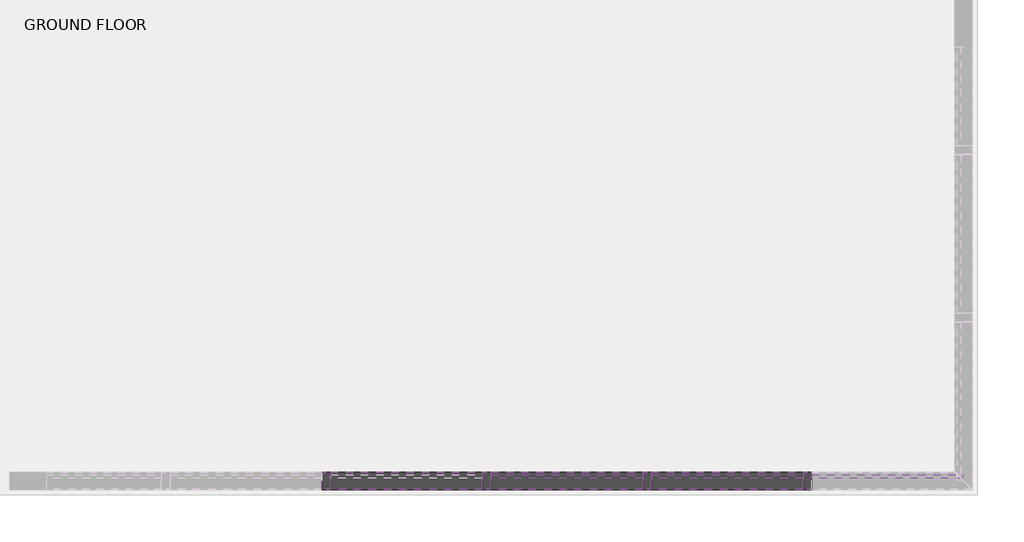
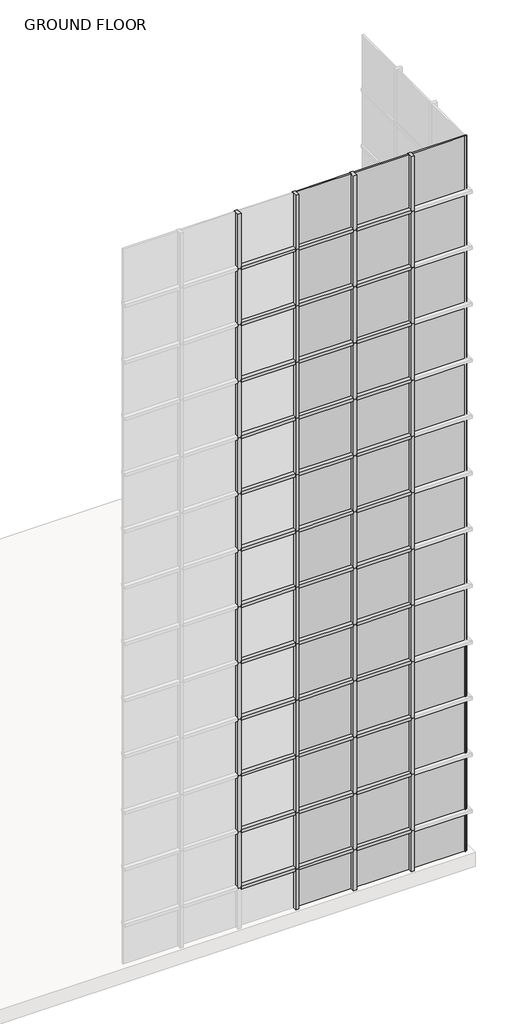
# One storey, part 5 of 16: 87 members, 43 plates.
"""IFC4 building model written with IfcOpenShell, lengths in millimetres."""

from ifc_helpers import new_model, si_unit, origin, place, context, project, spatial, transform, mapped, element, save
from components import member_d518c94e, member_b860638c, member_31fee25f, system_panel_glazed_5cba32e5, system_panel_glazed_49652e9e

model = new_model("IFC4")

# Units and contexts
model_context = context("Model", 3, world=origin())
ifc_project = project(units=[si_unit("LENGTHUNIT", "METRE", prefix="MILLI")], contexts=[model_context])

# Site, building, storey
site = spatial("IfcSite", under=ifc_project)
building = spatial("IfcBuilding", under=site)
storey = spatial("IfcBuildingStorey", under=building, Name="GROUND FLOOR", Elevation=0.0)

# Members
placement = place(None, origin())
member_shape = member_d518c94e(model_context)
element("IfcMember", 1, ObjectType="Rectangular Mullion : 2.5\" x 5\" rectangular", at=placement, inside=storey, context=model_context, shape_type="MappedRepresentation", body=[
    mapped(member_shape, transform((2466.2905541, -5739.2238032, 1168.8884615), x_axis=(0.0, 0.0, 1.0), y_axis=(0.0, -1.0, 0.0), z_axis=(1.0, 0.0, 0.0))),
])
element("IfcMember", 2, ObjectType="Rectangular Mullion : 2.5\" x 5\" rectangular", at=placement, inside=storey, context=model_context, shape_type="MappedRepresentation", body=[
    mapped(member_shape, transform((3631.7597848, -5739.2238032, 1168.8884615), x_axis=(0.0, 0.0, 1.0), y_axis=(0.0, -1.0, 0.0), z_axis=(1.0, 0.0, 0.0))),
])
element("IfcMember", 3, ObjectType="Rectangular Mullion : 2.5\" x 5\" rectangular", at=placement, inside=storey, context=model_context, shape_type="MappedRepresentation", body=[
    mapped(member_shape, transform((4797.2290155, -5739.2238032, 1168.8884615), x_axis=(0.0, 0.0, 1.0), y_axis=(0.0, -1.0, 0.0), z_axis=(1.0, 0.0, 0.0))),
])
element("IfcMember", 4, ObjectType="Rectangular Mullion : 2.5\" x 5\" rectangular", at=placement, inside=storey, context=model_context, shape_type="MappedRepresentation", body=[
    mapped(member_shape, transform((2466.2905541, -5739.2238032, 2369.5269231), x_axis=(0.0, 0.0, 1.0), y_axis=(0.0, -1.0, 0.0), z_axis=(1.0, 0.0, 0.0))),
])
element("IfcMember", 5, ObjectType="Rectangular Mullion : 2.5\" x 5\" rectangular", at=placement, inside=storey, context=model_context, shape_type="MappedRepresentation", body=[
    mapped(member_shape, transform((3631.7597848, -5739.2238032, 2369.5269231), x_axis=(0.0, 0.0, 1.0), y_axis=(0.0, -1.0, 0.0), z_axis=(1.0, 0.0, 0.0))),
])
element("IfcMember", 6, ObjectType="Rectangular Mullion : 2.5\" x 5\" rectangular", at=placement, inside=storey, context=model_context, shape_type="MappedRepresentation", body=[
    mapped(member_shape, transform((4797.2290155, -5739.2238032, 2369.5269231), x_axis=(0.0, 0.0, 1.0), y_axis=(0.0, -1.0, 0.0), z_axis=(1.0, 0.0, 0.0))),
])
element("IfcMember", 7, ObjectType="Rectangular Mullion : 2.5\" x 5\" rectangular", at=placement, inside=storey, context=model_context, shape_type="MappedRepresentation", body=[
    mapped(member_shape, transform((2466.2905541, -5739.2238032, 3570.1653846), x_axis=(0.0, 0.0, 1.0), y_axis=(0.0, -1.0, 0.0), z_axis=(1.0, 0.0, 0.0))),
])
element("IfcMember", 8, ObjectType="Rectangular Mullion : 2.5\" x 5\" rectangular", at=placement, inside=storey, context=model_context, shape_type="MappedRepresentation", body=[
    mapped(member_shape, transform((3631.7597848, -5739.2238032, 3570.1653846), x_axis=(0.0, 0.0, 1.0), y_axis=(0.0, -1.0, 0.0), z_axis=(1.0, 0.0, 0.0))),
])
element("IfcMember", 9, ObjectType="Rectangular Mullion : 2.5\" x 5\" rectangular", at=placement, inside=storey, context=model_context, shape_type="MappedRepresentation", body=[
    mapped(member_shape, transform((4797.2290155, -5739.2238032, 3570.1653846), x_axis=(0.0, 0.0, 1.0), y_axis=(0.0, -1.0, 0.0), z_axis=(1.0, 0.0, 0.0))),
])
element("IfcMember", 10, ObjectType="Rectangular Mullion : 2.5\" x 5\" rectangular", at=placement, inside=storey, context=model_context, shape_type="MappedRepresentation", body=[
    mapped(member_shape, transform((2466.2905541, -5739.2238032, 4770.8038462), x_axis=(0.0, 0.0, 1.0), y_axis=(0.0, -1.0, 0.0), z_axis=(1.0, 0.0, 0.0))),
])
element("IfcMember", 11, ObjectType="Rectangular Mullion : 2.5\" x 5\" rectangular", at=placement, inside=storey, context=model_context, shape_type="MappedRepresentation", body=[
    mapped(member_shape, transform((3631.7597848, -5739.2238032, 4770.8038462), x_axis=(0.0, 0.0, 1.0), y_axis=(0.0, -1.0, 0.0), z_axis=(1.0, 0.0, 0.0))),
])
element("IfcMember", 12, ObjectType="Rectangular Mullion : 2.5\" x 5\" rectangular", at=placement, inside=storey, context=model_context, shape_type="MappedRepresentation", body=[
    mapped(member_shape, transform((4797.2290155, -5739.2238032, 4770.8038462), x_axis=(0.0, 0.0, 1.0), y_axis=(0.0, -1.0, 0.0), z_axis=(1.0, 0.0, 0.0))),
])
element("IfcMember", 13, ObjectType="Rectangular Mullion : 2.5\" x 5\" rectangular", at=placement, inside=storey, context=model_context, shape_type="MappedRepresentation", body=[
    mapped(member_shape, transform((2466.2905541, -5739.2238032, 5971.4423077), x_axis=(0.0, 0.0, 1.0), y_axis=(0.0, -1.0, 0.0), z_axis=(1.0, 0.0, 0.0))),
])
element("IfcMember", 14, ObjectType="Rectangular Mullion : 2.5\" x 5\" rectangular", at=placement, inside=storey, context=model_context, shape_type="MappedRepresentation", body=[
    mapped(member_shape, transform((3631.7597848, -5739.2238032, 5971.4423077), x_axis=(0.0, 0.0, 1.0), y_axis=(0.0, -1.0, 0.0), z_axis=(1.0, 0.0, 0.0))),
])
element("IfcMember", 15, ObjectType="Rectangular Mullion : 2.5\" x 5\" rectangular", at=placement, inside=storey, context=model_context, shape_type="MappedRepresentation", body=[
    mapped(member_shape, transform((4797.2290155, -5739.2238032, 5971.4423077), x_axis=(0.0, 0.0, 1.0), y_axis=(0.0, -1.0, 0.0), z_axis=(1.0, 0.0, 0.0))),
])
element("IfcMember", 16, ObjectType="Rectangular Mullion : 2.5\" x 5\" rectangular", at=placement, inside=storey, context=model_context, shape_type="MappedRepresentation", body=[
    mapped(member_shape, transform((2466.2905541, -5739.2238032, 7172.0807692), x_axis=(0.0, 0.0, 1.0), y_axis=(0.0, -1.0, 0.0), z_axis=(1.0, 0.0, 0.0))),
])
element("IfcMember", 17, ObjectType="Rectangular Mullion : 2.5\" x 5\" rectangular", at=placement, inside=storey, context=model_context, shape_type="MappedRepresentation", body=[
    mapped(member_shape, transform((3631.7597848, -5739.2238032, 7172.0807692), x_axis=(0.0, 0.0, 1.0), y_axis=(0.0, -1.0, 0.0), z_axis=(1.0, 0.0, 0.0))),
])
element("IfcMember", 18, ObjectType="Rectangular Mullion : 2.5\" x 5\" rectangular", at=placement, inside=storey, context=model_context, shape_type="MappedRepresentation", body=[
    mapped(member_shape, transform((4797.2290155, -5739.2238032, 7172.0807692), x_axis=(0.0, 0.0, 1.0), y_axis=(0.0, -1.0, 0.0), z_axis=(1.0, 0.0, 0.0))),
])
element("IfcMember", 19, ObjectType="Rectangular Mullion : 2.5\" x 5\" rectangular", at=placement, inside=storey, context=model_context, shape_type="MappedRepresentation", body=[
    mapped(member_shape, transform((2466.2905541, -5739.2238032, 8372.7192308), x_axis=(0.0, 0.0, 1.0), y_axis=(0.0, -1.0, 0.0), z_axis=(1.0, 0.0, 0.0))),
])
element("IfcMember", 20, ObjectType="Rectangular Mullion : 2.5\" x 5\" rectangular", at=placement, inside=storey, context=model_context, shape_type="MappedRepresentation", body=[
    mapped(member_shape, transform((3631.7597848, -5739.2238032, 8372.7192308), x_axis=(0.0, 0.0, 1.0), y_axis=(0.0, -1.0, 0.0), z_axis=(1.0, 0.0, 0.0))),
])
element("IfcMember", 21, ObjectType="Rectangular Mullion : 2.5\" x 5\" rectangular", at=placement, inside=storey, context=model_context, shape_type="MappedRepresentation", body=[
    mapped(member_shape, transform((4797.2290155, -5739.2238032, 8372.7192308), x_axis=(0.0, 0.0, 1.0), y_axis=(0.0, -1.0, 0.0), z_axis=(1.0, 0.0, 0.0))),
])
element("IfcMember", 22, ObjectType="Rectangular Mullion : 2.5\" x 5\" rectangular", at=placement, inside=storey, context=model_context, shape_type="MappedRepresentation", body=[
    mapped(member_shape, transform((2466.2905541, -5739.2238032, 9573.3576923), x_axis=(0.0, 0.0, 1.0), y_axis=(0.0, -1.0, 0.0), z_axis=(1.0, 0.0, 0.0))),
])
element("IfcMember", 23, ObjectType="Rectangular Mullion : 2.5\" x 5\" rectangular", at=placement, inside=storey, context=model_context, shape_type="MappedRepresentation", body=[
    mapped(member_shape, transform((3631.7597848, -5739.2238032, 9573.3576923), x_axis=(0.0, 0.0, 1.0), y_axis=(0.0, -1.0, 0.0), z_axis=(1.0, 0.0, 0.0))),
])
element("IfcMember", 24, ObjectType="Rectangular Mullion : 2.5\" x 5\" rectangular", at=placement, inside=storey, context=model_context, shape_type="MappedRepresentation", body=[
    mapped(member_shape, transform((4797.2290155, -5739.2238032, 9573.3576923), x_axis=(0.0, 0.0, 1.0), y_axis=(0.0, -1.0, 0.0), z_axis=(1.0, 0.0, 0.0))),
])
element("IfcMember", 25, ObjectType="Rectangular Mullion : 2.5\" x 5\" rectangular", at=placement, inside=storey, context=model_context, shape_type="MappedRepresentation", body=[
    mapped(member_shape, transform((2466.2905541, -5739.2238032, 10773.9961538), x_axis=(0.0, 0.0, 1.0), y_axis=(0.0, -1.0, 0.0), z_axis=(1.0, 0.0, 0.0))),
])
element("IfcMember", 26, ObjectType="Rectangular Mullion : 2.5\" x 5\" rectangular", at=placement, inside=storey, context=model_context, shape_type="MappedRepresentation", body=[
    mapped(member_shape, transform((3631.7597848, -5739.2238032, 10773.9961538), x_axis=(0.0, 0.0, 1.0), y_axis=(0.0, -1.0, 0.0), z_axis=(1.0, 0.0, 0.0))),
])
element("IfcMember", 27, ObjectType="Rectangular Mullion : 2.5\" x 5\" rectangular", at=placement, inside=storey, context=model_context, shape_type="MappedRepresentation", body=[
    mapped(member_shape, transform((4797.2290155, -5739.2238032, 10773.9961538), x_axis=(0.0, 0.0, 1.0), y_axis=(0.0, -1.0, 0.0), z_axis=(1.0, 0.0, 0.0))),
])
element("IfcMember", 28, ObjectType="Rectangular Mullion : 2.5\" x 5\" rectangular", at=placement, inside=storey, context=model_context, shape_type="MappedRepresentation", body=[
    mapped(member_shape, transform((2466.2905541, -5739.2238032, 11974.6346154), x_axis=(0.0, 0.0, 1.0), y_axis=(0.0, -1.0, 0.0), z_axis=(1.0, 0.0, 0.0))),
])
element("IfcMember", 29, ObjectType="Rectangular Mullion : 2.5\" x 5\" rectangular", at=placement, inside=storey, context=model_context, shape_type="MappedRepresentation", body=[
    mapped(member_shape, transform((3631.7597848, -5739.2238032, 11974.6346154), x_axis=(0.0, 0.0, 1.0), y_axis=(0.0, -1.0, 0.0), z_axis=(1.0, 0.0, 0.0))),
])
element("IfcMember", 30, ObjectType="Rectangular Mullion : 2.5\" x 5\" rectangular", at=placement, inside=storey, context=model_context, shape_type="MappedRepresentation", body=[
    mapped(member_shape, transform((4797.2290155, -5739.2238032, 11974.6346154), x_axis=(0.0, 0.0, 1.0), y_axis=(0.0, -1.0, 0.0), z_axis=(1.0, 0.0, 0.0))),
])
element("IfcMember", 31, ObjectType="Rectangular Mullion : 2.5\" x 5\" rectangular", at=placement, inside=storey, context=model_context, shape_type="MappedRepresentation", body=[
    mapped(member_shape, transform((2466.2905541, -5739.2238032, 13175.2730769), x_axis=(0.0, 0.0, 1.0), y_axis=(0.0, -1.0, 0.0), z_axis=(1.0, 0.0, 0.0))),
])
element("IfcMember", 32, ObjectType="Rectangular Mullion : 2.5\" x 5\" rectangular", at=placement, inside=storey, context=model_context, shape_type="MappedRepresentation", body=[
    mapped(member_shape, transform((3631.7597848, -5739.2238032, 13175.2730769), x_axis=(0.0, 0.0, 1.0), y_axis=(0.0, -1.0, 0.0), z_axis=(1.0, 0.0, 0.0))),
])
element("IfcMember", 33, ObjectType="Rectangular Mullion : 2.5\" x 5\" rectangular", at=placement, inside=storey, context=model_context, shape_type="MappedRepresentation", body=[
    mapped(member_shape, transform((4797.2290155, -5739.2238032, 13175.2730769), x_axis=(0.0, 0.0, 1.0), y_axis=(0.0, -1.0, 0.0), z_axis=(1.0, 0.0, 0.0))),
])
element("IfcMember", 34, ObjectType="Rectangular Mullion : 2.5\" x 5\" rectangular", at=placement, inside=storey, context=model_context, shape_type="MappedRepresentation", body=[
    mapped(member_shape, transform((2466.2905541, -5739.2238032, 14375.9115385), x_axis=(0.0, 0.0, 1.0), y_axis=(0.0, -1.0, 0.0), z_axis=(1.0, 0.0, 0.0))),
])
element("IfcMember", 35, ObjectType="Rectangular Mullion : 2.5\" x 5\" rectangular", at=placement, inside=storey, context=model_context, shape_type="MappedRepresentation", body=[
    mapped(member_shape, transform((3631.7597848, -5739.2238032, 14375.9115385), x_axis=(0.0, 0.0, 1.0), y_axis=(0.0, -1.0, 0.0), z_axis=(1.0, 0.0, 0.0))),
])
element("IfcMember", 36, ObjectType="Rectangular Mullion : 2.5\" x 5\" rectangular", at=placement, inside=storey, context=model_context, shape_type="MappedRepresentation", body=[
    mapped(member_shape, transform((4797.2290155, -5739.2238032, 14375.9115385), x_axis=(0.0, 0.0, 1.0), y_axis=(0.0, -1.0, 0.0), z_axis=(1.0, 0.0, 0.0))),
])
member_2_shape = member_b860638c(model_context)
element("IfcMember", 37, ObjectType="Rectangular Mullion : 2.5\" x 5\" rectangular", at=placement, inside=storey, context=model_context, shape_type="MappedRepresentation", body=[
    mapped(member_2_shape, transform((2498.0405541, -5739.2238032, 0.0), x_axis=(1.0, 0.0, 0.0), y_axis=(0.0, -1.0, 0.0), z_axis=(0.0, 0.0, -1.0))),
])
element("IfcMember", 38, ObjectType="Rectangular Mullion : 2.5\" x 5\" rectangular", at=placement, inside=storey, context=model_context, shape_type="MappedRepresentation", body=[
    mapped(member_2_shape, transform((3663.5097848, -5739.2238032, 0.0), x_axis=(1.0, 0.0, 0.0), y_axis=(0.0, -1.0, 0.0), z_axis=(0.0, 0.0, -1.0))),
])
element("IfcMember", 39, ObjectType="Rectangular Mullion : 2.5\" x 5\" rectangular", at=placement, inside=storey, context=model_context, shape_type="MappedRepresentation", body=[
    mapped(member_2_shape, transform((4828.9790155, -5739.2238032, 0.0), x_axis=(1.0, 0.0, 0.0), y_axis=(0.0, -1.0, 0.0), z_axis=(0.0, 0.0, -1.0))),
])
member_3_shape = member_31fee25f(model_context)
element("IfcMember", 40, ObjectType="Rectangular Mullion : 2.5\" x 5\" rectangular", at=placement, inside=storey, context=model_context, shape_type="MappedRepresentation", body=[
    mapped(member_3_shape, transform((1332.5713234, -5739.2238032, 1168.8884615), x_axis=(1.0, 0.0, 0.0), y_axis=(0.0, -1.0, 0.0), z_axis=(0.0, 0.0, -1.0))),
])
element("IfcMember", 41, ObjectType="Rectangular Mullion : 2.5\" x 5\" rectangular", at=placement, inside=storey, context=model_context, shape_type="MappedRepresentation", body=[
    mapped(member_3_shape, transform((2498.0405541, -5739.2238032, 1168.8884615), x_axis=(1.0, 0.0, 0.0), y_axis=(0.0, -1.0, 0.0), z_axis=(0.0, 0.0, -1.0))),
])
element("IfcMember", 42, ObjectType="Rectangular Mullion : 2.5\" x 5\" rectangular", at=placement, inside=storey, context=model_context, shape_type="MappedRepresentation", body=[
    mapped(member_3_shape, transform((3663.5097848, -5739.2238032, 1168.8884615), x_axis=(1.0, 0.0, 0.0), y_axis=(0.0, -1.0, 0.0), z_axis=(0.0, 0.0, -1.0))),
])
element("IfcMember", 43, ObjectType="Rectangular Mullion : 2.5\" x 5\" rectangular", at=placement, inside=storey, context=model_context, shape_type="MappedRepresentation", body=[
    mapped(member_3_shape, transform((4828.9790155, -5739.2238032, 1168.8884615), x_axis=(1.0, 0.0, 0.0), y_axis=(0.0, -1.0, 0.0), z_axis=(0.0, 0.0, -1.0))),
])
element("IfcMember", 44, ObjectType="Rectangular Mullion : 2.5\" x 5\" rectangular", at=placement, inside=storey, context=model_context, shape_type="MappedRepresentation", body=[
    mapped(member_3_shape, transform((1332.5713234, -5739.2238032, 2369.5269231), x_axis=(1.0, 0.0, 0.0), y_axis=(0.0, -1.0, 0.0), z_axis=(0.0, 0.0, -1.0))),
])
element("IfcMember", 45, ObjectType="Rectangular Mullion : 2.5\" x 5\" rectangular", at=placement, inside=storey, context=model_context, shape_type="MappedRepresentation", body=[
    mapped(member_3_shape, transform((2498.0405541, -5739.2238032, 2369.5269231), x_axis=(1.0, 0.0, 0.0), y_axis=(0.0, -1.0, 0.0), z_axis=(0.0, 0.0, -1.0))),
])
element("IfcMember", 46, ObjectType="Rectangular Mullion : 2.5\" x 5\" rectangular", at=placement, inside=storey, context=model_context, shape_type="MappedRepresentation", body=[
    mapped(member_3_shape, transform((3663.5097848, -5739.2238032, 2369.5269231), x_axis=(1.0, 0.0, 0.0), y_axis=(0.0, -1.0, 0.0), z_axis=(0.0, 0.0, -1.0))),
])
element("IfcMember", 47, ObjectType="Rectangular Mullion : 2.5\" x 5\" rectangular", at=placement, inside=storey, context=model_context, shape_type="MappedRepresentation", body=[
    mapped(member_3_shape, transform((4828.9790155, -5739.2238032, 2369.5269231), x_axis=(1.0, 0.0, 0.0), y_axis=(0.0, -1.0, 0.0), z_axis=(0.0, 0.0, -1.0))),
])
element("IfcMember", 48, ObjectType="Rectangular Mullion : 2.5\" x 5\" rectangular", at=placement, inside=storey, context=model_context, shape_type="MappedRepresentation", body=[
    mapped(member_3_shape, transform((1332.5713234, -5739.2238032, 3570.1653846), x_axis=(1.0, 0.0, 0.0), y_axis=(0.0, -1.0, 0.0), z_axis=(0.0, 0.0, -1.0))),
])
element("IfcMember", 49, ObjectType="Rectangular Mullion : 2.5\" x 5\" rectangular", at=placement, inside=storey, context=model_context, shape_type="MappedRepresentation", body=[
    mapped(member_3_shape, transform((2498.0405541, -5739.2238032, 3570.1653846), x_axis=(1.0, 0.0, 0.0), y_axis=(0.0, -1.0, 0.0), z_axis=(0.0, 0.0, -1.0))),
])
element("IfcMember", 50, ObjectType="Rectangular Mullion : 2.5\" x 5\" rectangular", at=placement, inside=storey, context=model_context, shape_type="MappedRepresentation", body=[
    mapped(member_3_shape, transform((3663.5097848, -5739.2238032, 3570.1653846), x_axis=(1.0, 0.0, 0.0), y_axis=(0.0, -1.0, 0.0), z_axis=(0.0, 0.0, -1.0))),
])
element("IfcMember", 51, ObjectType="Rectangular Mullion : 2.5\" x 5\" rectangular", at=placement, inside=storey, context=model_context, shape_type="MappedRepresentation", body=[
    mapped(member_3_shape, transform((4828.9790155, -5739.2238032, 3570.1653846), x_axis=(1.0, 0.0, 0.0), y_axis=(0.0, -1.0, 0.0), z_axis=(0.0, 0.0, -1.0))),
])
element("IfcMember", 52, ObjectType="Rectangular Mullion : 2.5\" x 5\" rectangular", at=placement, inside=storey, context=model_context, shape_type="MappedRepresentation", body=[
    mapped(member_3_shape, transform((1332.5713234, -5739.2238032, 4770.8038462), x_axis=(1.0, 0.0, 0.0), y_axis=(0.0, -1.0, 0.0), z_axis=(0.0, 0.0, -1.0))),
])
element("IfcMember", 53, ObjectType="Rectangular Mullion : 2.5\" x 5\" rectangular", at=placement, inside=storey, context=model_context, shape_type="MappedRepresentation", body=[
    mapped(member_3_shape, transform((2498.0405541, -5739.2238032, 4770.8038462), x_axis=(1.0, 0.0, 0.0), y_axis=(0.0, -1.0, 0.0), z_axis=(0.0, 0.0, -1.0))),
])
element("IfcMember", 54, ObjectType="Rectangular Mullion : 2.5\" x 5\" rectangular", at=placement, inside=storey, context=model_context, shape_type="MappedRepresentation", body=[
    mapped(member_3_shape, transform((3663.5097848, -5739.2238032, 4770.8038462), x_axis=(1.0, 0.0, 0.0), y_axis=(0.0, -1.0, 0.0), z_axis=(0.0, 0.0, -1.0))),
])
element("IfcMember", 55, ObjectType="Rectangular Mullion : 2.5\" x 5\" rectangular", at=placement, inside=storey, context=model_context, shape_type="MappedRepresentation", body=[
    mapped(member_3_shape, transform((4828.9790155, -5739.2238032, 4770.8038462), x_axis=(1.0, 0.0, 0.0), y_axis=(0.0, -1.0, 0.0), z_axis=(0.0, 0.0, -1.0))),
])
element("IfcMember", 56, ObjectType="Rectangular Mullion : 2.5\" x 5\" rectangular", at=placement, inside=storey, context=model_context, shape_type="MappedRepresentation", body=[
    mapped(member_3_shape, transform((1332.5713234, -5739.2238032, 5971.4423077), x_axis=(1.0, 0.0, 0.0), y_axis=(0.0, -1.0, 0.0), z_axis=(0.0, 0.0, -1.0))),
])
element("IfcMember", 57, ObjectType="Rectangular Mullion : 2.5\" x 5\" rectangular", at=placement, inside=storey, context=model_context, shape_type="MappedRepresentation", body=[
    mapped(member_3_shape, transform((2498.0405541, -5739.2238032, 5971.4423077), x_axis=(1.0, 0.0, 0.0), y_axis=(0.0, -1.0, 0.0), z_axis=(0.0, 0.0, -1.0))),
])
element("IfcMember", 58, ObjectType="Rectangular Mullion : 2.5\" x 5\" rectangular", at=placement, inside=storey, context=model_context, shape_type="MappedRepresentation", body=[
    mapped(member_3_shape, transform((3663.5097848, -5739.2238032, 5971.4423077), x_axis=(1.0, 0.0, 0.0), y_axis=(0.0, -1.0, 0.0), z_axis=(0.0, 0.0, -1.0))),
])
element("IfcMember", 59, ObjectType="Rectangular Mullion : 2.5\" x 5\" rectangular", at=placement, inside=storey, context=model_context, shape_type="MappedRepresentation", body=[
    mapped(member_3_shape, transform((4828.9790155, -5739.2238032, 5971.4423077), x_axis=(1.0, 0.0, 0.0), y_axis=(0.0, -1.0, 0.0), z_axis=(0.0, 0.0, -1.0))),
])
element("IfcMember", 60, ObjectType="Rectangular Mullion : 2.5\" x 5\" rectangular", at=placement, inside=storey, context=model_context, shape_type="MappedRepresentation", body=[
    mapped(member_3_shape, transform((1332.5713234, -5739.2238032, 7172.0807692), x_axis=(1.0, 0.0, 0.0), y_axis=(0.0, -1.0, 0.0), z_axis=(0.0, 0.0, -1.0))),
])
element("IfcMember", 61, ObjectType="Rectangular Mullion : 2.5\" x 5\" rectangular", at=placement, inside=storey, context=model_context, shape_type="MappedRepresentation", body=[
    mapped(member_3_shape, transform((2498.0405541, -5739.2238032, 7172.0807692), x_axis=(1.0, 0.0, 0.0), y_axis=(0.0, -1.0, 0.0), z_axis=(0.0, 0.0, -1.0))),
])
element("IfcMember", 62, ObjectType="Rectangular Mullion : 2.5\" x 5\" rectangular", at=placement, inside=storey, context=model_context, shape_type="MappedRepresentation", body=[
    mapped(member_3_shape, transform((3663.5097848, -5739.2238032, 7172.0807692), x_axis=(1.0, 0.0, 0.0), y_axis=(0.0, -1.0, 0.0), z_axis=(0.0, 0.0, -1.0))),
])
element("IfcMember", 63, ObjectType="Rectangular Mullion : 2.5\" x 5\" rectangular", at=placement, inside=storey, context=model_context, shape_type="MappedRepresentation", body=[
    mapped(member_3_shape, transform((4828.9790155, -5739.2238032, 7172.0807692), x_axis=(1.0, 0.0, 0.0), y_axis=(0.0, -1.0, 0.0), z_axis=(0.0, 0.0, -1.0))),
])
element("IfcMember", 64, ObjectType="Rectangular Mullion : 2.5\" x 5\" rectangular", at=placement, inside=storey, context=model_context, shape_type="MappedRepresentation", body=[
    mapped(member_3_shape, transform((1332.5713234, -5739.2238032, 8372.7192308), x_axis=(1.0, 0.0, 0.0), y_axis=(0.0, -1.0, 0.0), z_axis=(0.0, 0.0, -1.0))),
])
element("IfcMember", 65, ObjectType="Rectangular Mullion : 2.5\" x 5\" rectangular", at=placement, inside=storey, context=model_context, shape_type="MappedRepresentation", body=[
    mapped(member_3_shape, transform((2498.0405541, -5739.2238032, 8372.7192308), x_axis=(1.0, 0.0, 0.0), y_axis=(0.0, -1.0, 0.0), z_axis=(0.0, 0.0, -1.0))),
])
element("IfcMember", 66, ObjectType="Rectangular Mullion : 2.5\" x 5\" rectangular", at=placement, inside=storey, context=model_context, shape_type="MappedRepresentation", body=[
    mapped(member_3_shape, transform((3663.5097848, -5739.2238032, 8372.7192308), x_axis=(1.0, 0.0, 0.0), y_axis=(0.0, -1.0, 0.0), z_axis=(0.0, 0.0, -1.0))),
])
element("IfcMember", 67, ObjectType="Rectangular Mullion : 2.5\" x 5\" rectangular", at=placement, inside=storey, context=model_context, shape_type="MappedRepresentation", body=[
    mapped(member_3_shape, transform((4828.9790155, -5739.2238032, 8372.7192308), x_axis=(1.0, 0.0, 0.0), y_axis=(0.0, -1.0, 0.0), z_axis=(0.0, 0.0, -1.0))),
])
element("IfcMember", 68, ObjectType="Rectangular Mullion : 2.5\" x 5\" rectangular", at=placement, inside=storey, context=model_context, shape_type="MappedRepresentation", body=[
    mapped(member_3_shape, transform((1332.5713234, -5739.2238032, 9573.3576923), x_axis=(1.0, 0.0, 0.0), y_axis=(0.0, -1.0, 0.0), z_axis=(0.0, 0.0, -1.0))),
])
element("IfcMember", 69, ObjectType="Rectangular Mullion : 2.5\" x 5\" rectangular", at=placement, inside=storey, context=model_context, shape_type="MappedRepresentation", body=[
    mapped(member_3_shape, transform((2498.0405541, -5739.2238032, 9573.3576923), x_axis=(1.0, 0.0, 0.0), y_axis=(0.0, -1.0, 0.0), z_axis=(0.0, 0.0, -1.0))),
])
element("IfcMember", 70, ObjectType="Rectangular Mullion : 2.5\" x 5\" rectangular", at=placement, inside=storey, context=model_context, shape_type="MappedRepresentation", body=[
    mapped(member_3_shape, transform((3663.5097848, -5739.2238032, 9573.3576923), x_axis=(1.0, 0.0, 0.0), y_axis=(0.0, -1.0, 0.0), z_axis=(0.0, 0.0, -1.0))),
])
element("IfcMember", 71, ObjectType="Rectangular Mullion : 2.5\" x 5\" rectangular", at=placement, inside=storey, context=model_context, shape_type="MappedRepresentation", body=[
    mapped(member_3_shape, transform((4828.9790155, -5739.2238032, 9573.3576923), x_axis=(1.0, 0.0, 0.0), y_axis=(0.0, -1.0, 0.0), z_axis=(0.0, 0.0, -1.0))),
])
element("IfcMember", 72, ObjectType="Rectangular Mullion : 2.5\" x 5\" rectangular", at=placement, inside=storey, context=model_context, shape_type="MappedRepresentation", body=[
    mapped(member_3_shape, transform((1332.5713234, -5739.2238032, 10773.9961538), x_axis=(1.0, 0.0, 0.0), y_axis=(0.0, -1.0, 0.0), z_axis=(0.0, 0.0, -1.0))),
])
element("IfcMember", 73, ObjectType="Rectangular Mullion : 2.5\" x 5\" rectangular", at=placement, inside=storey, context=model_context, shape_type="MappedRepresentation", body=[
    mapped(member_3_shape, transform((2498.0405541, -5739.2238032, 10773.9961538), x_axis=(1.0, 0.0, 0.0), y_axis=(0.0, -1.0, 0.0), z_axis=(0.0, 0.0, -1.0))),
])
element("IfcMember", 74, ObjectType="Rectangular Mullion : 2.5\" x 5\" rectangular", at=placement, inside=storey, context=model_context, shape_type="MappedRepresentation", body=[
    mapped(member_3_shape, transform((3663.5097848, -5739.2238032, 10773.9961538), x_axis=(1.0, 0.0, 0.0), y_axis=(0.0, -1.0, 0.0), z_axis=(0.0, 0.0, -1.0))),
])
element("IfcMember", 75, ObjectType="Rectangular Mullion : 2.5\" x 5\" rectangular", at=placement, inside=storey, context=model_context, shape_type="MappedRepresentation", body=[
    mapped(member_3_shape, transform((4828.9790155, -5739.2238032, 10773.9961538), x_axis=(1.0, 0.0, 0.0), y_axis=(0.0, -1.0, 0.0), z_axis=(0.0, 0.0, -1.0))),
])
element("IfcMember", 76, ObjectType="Rectangular Mullion : 2.5\" x 5\" rectangular", at=placement, inside=storey, context=model_context, shape_type="MappedRepresentation", body=[
    mapped(member_3_shape, transform((1332.5713234, -5739.2238032, 11974.6346154), x_axis=(1.0, 0.0, 0.0), y_axis=(0.0, -1.0, 0.0), z_axis=(0.0, 0.0, -1.0))),
])
element("IfcMember", 77, ObjectType="Rectangular Mullion : 2.5\" x 5\" rectangular", at=placement, inside=storey, context=model_context, shape_type="MappedRepresentation", body=[
    mapped(member_3_shape, transform((2498.0405541, -5739.2238032, 11974.6346154), x_axis=(1.0, 0.0, 0.0), y_axis=(0.0, -1.0, 0.0), z_axis=(0.0, 0.0, -1.0))),
])
element("IfcMember", 78, ObjectType="Rectangular Mullion : 2.5\" x 5\" rectangular", at=placement, inside=storey, context=model_context, shape_type="MappedRepresentation", body=[
    mapped(member_3_shape, transform((3663.5097848, -5739.2238032, 11974.6346154), x_axis=(1.0, 0.0, 0.0), y_axis=(0.0, -1.0, 0.0), z_axis=(0.0, 0.0, -1.0))),
])
element("IfcMember", 79, ObjectType="Rectangular Mullion : 2.5\" x 5\" rectangular", at=placement, inside=storey, context=model_context, shape_type="MappedRepresentation", body=[
    mapped(member_3_shape, transform((4828.9790155, -5739.2238032, 11974.6346154), x_axis=(1.0, 0.0, 0.0), y_axis=(0.0, -1.0, 0.0), z_axis=(0.0, 0.0, -1.0))),
])
element("IfcMember", 80, ObjectType="Rectangular Mullion : 2.5\" x 5\" rectangular", at=placement, inside=storey, context=model_context, shape_type="MappedRepresentation", body=[
    mapped(member_3_shape, transform((1332.5713234, -5739.2238032, 13175.2730769), x_axis=(1.0, 0.0, 0.0), y_axis=(0.0, -1.0, 0.0), z_axis=(0.0, 0.0, -1.0))),
])
element("IfcMember", 81, ObjectType="Rectangular Mullion : 2.5\" x 5\" rectangular", at=placement, inside=storey, context=model_context, shape_type="MappedRepresentation", body=[
    mapped(member_3_shape, transform((2498.0405541, -5739.2238032, 13175.2730769), x_axis=(1.0, 0.0, 0.0), y_axis=(0.0, -1.0, 0.0), z_axis=(0.0, 0.0, -1.0))),
])
element("IfcMember", 82, ObjectType="Rectangular Mullion : 2.5\" x 5\" rectangular", at=placement, inside=storey, context=model_context, shape_type="MappedRepresentation", body=[
    mapped(member_3_shape, transform((3663.5097848, -5739.2238032, 13175.2730769), x_axis=(1.0, 0.0, 0.0), y_axis=(0.0, -1.0, 0.0), z_axis=(0.0, 0.0, -1.0))),
])
element("IfcMember", 83, ObjectType="Rectangular Mullion : 2.5\" x 5\" rectangular", at=placement, inside=storey, context=model_context, shape_type="MappedRepresentation", body=[
    mapped(member_3_shape, transform((4828.9790155, -5739.2238032, 13175.2730769), x_axis=(1.0, 0.0, 0.0), y_axis=(0.0, -1.0, 0.0), z_axis=(0.0, 0.0, -1.0))),
])
element("IfcMember", 84, ObjectType="Rectangular Mullion : 2.5\" x 5\" rectangular", at=placement, inside=storey, context=model_context, shape_type="MappedRepresentation", body=[
    mapped(member_2_shape, transform((1332.5713234, -5739.2238032, 14375.9115385), x_axis=(1.0, 0.0, 0.0), y_axis=(0.0, -1.0, 0.0), z_axis=(0.0, 0.0, -1.0))),
])
element("IfcMember", 85, ObjectType="Rectangular Mullion : 2.5\" x 5\" rectangular", at=placement, inside=storey, context=model_context, shape_type="MappedRepresentation", body=[
    mapped(member_2_shape, transform((2498.0405541, -5739.2238032, 14375.9115385), x_axis=(1.0, 0.0, 0.0), y_axis=(0.0, -1.0, 0.0), z_axis=(0.0, 0.0, -1.0))),
])
element("IfcMember", 86, ObjectType="Rectangular Mullion : 2.5\" x 5\" rectangular", at=placement, inside=storey, context=model_context, shape_type="MappedRepresentation", body=[
    mapped(member_2_shape, transform((3663.5097848, -5739.2238032, 14375.9115385), x_axis=(1.0, 0.0, 0.0), y_axis=(0.0, -1.0, 0.0), z_axis=(0.0, 0.0, -1.0))),
])
element("IfcMember", 87, ObjectType="Rectangular Mullion : 2.5\" x 5\" rectangular", at=placement, inside=storey, context=model_context, shape_type="MappedRepresentation", body=[
    mapped(member_2_shape, transform((4828.9790155, -5739.2238032, 14375.9115385), x_axis=(1.0, 0.0, 0.0), y_axis=(0.0, -1.0, 0.0), z_axis=(0.0, 0.0, -1.0))),
])

# Plates
system_panel_glazed_shape = system_panel_glazed_5cba32e5(model_context)
element("IfcPlate", 88, ObjectType="System Panel : Glazed", at=placement, inside=storey, context=model_context, shape_type="MappedRepresentation", body=[
    mapped(system_panel_glazed_shape, transform((3080.7751695, -5739.2238032, 0.0), x_axis=(1.0, 0.0, 0.0), y_axis=(0.0, 1.0, 0.0), z_axis=(0.0, 0.0, 1.0))),
])
element("IfcPlate", 89, ObjectType="System Panel : Glazed", at=placement, inside=storey, context=model_context, shape_type="MappedRepresentation", body=[
    mapped(system_panel_glazed_shape, transform((4246.2444002, -5739.2238032, 0.0), x_axis=(1.0, 0.0, 0.0), y_axis=(0.0, 1.0, 0.0), z_axis=(0.0, 0.0, 1.0))),
])
element("IfcPlate", 90, ObjectType="System Panel : Glazed", at=placement, inside=storey, context=model_context, shape_type="MappedRepresentation", body=[
    mapped(system_panel_glazed_shape, transform((5411.7136311, -5739.2238032, 0.0), x_axis=(1.0, 0.0, 0.0), y_axis=(0.0, 1.0, 0.0), z_axis=(0.0, 0.0, 1.0))),
])
element("IfcPlate", 91, ObjectType="System Panel : Glazed", at=placement, inside=storey, context=model_context, shape_type="MappedRepresentation", body=[
    mapped(system_panel_glazed_shape, transform((3080.7751695, -5739.2238032, 1200.6384615), x_axis=(1.0, 0.0, 0.0), y_axis=(0.0, 1.0, 0.0), z_axis=(0.0, 0.0, 1.0))),
])
element("IfcPlate", 92, ObjectType="System Panel : Glazed", at=placement, inside=storey, context=model_context, shape_type="MappedRepresentation", body=[
    mapped(system_panel_glazed_shape, transform((4246.2444002, -5739.2238032, 1200.6384615), x_axis=(1.0, 0.0, 0.0), y_axis=(0.0, 1.0, 0.0), z_axis=(0.0, 0.0, 1.0))),
])
element("IfcPlate", 93, ObjectType="System Panel : Glazed", at=placement, inside=storey, context=model_context, shape_type="MappedRepresentation", body=[
    mapped(system_panel_glazed_shape, transform((5411.7136311, -5739.2238032, 1200.6384615), x_axis=(1.0, 0.0, 0.0), y_axis=(0.0, 1.0, 0.0), z_axis=(0.0, 0.0, 1.0))),
])
element("IfcPlate", 94, ObjectType="System Panel : Glazed", at=placement, inside=storey, context=model_context, shape_type="MappedRepresentation", body=[
    mapped(system_panel_glazed_shape, transform((3080.7751695, -5739.2238032, 2401.2769231), x_axis=(1.0, 0.0, 0.0), y_axis=(0.0, 1.0, 0.0), z_axis=(0.0, 0.0, 1.0))),
])
element("IfcPlate", 95, ObjectType="System Panel : Glazed", at=placement, inside=storey, context=model_context, shape_type="MappedRepresentation", body=[
    mapped(system_panel_glazed_shape, transform((4246.2444002, -5739.2238032, 2401.2769231), x_axis=(1.0, 0.0, 0.0), y_axis=(0.0, 1.0, 0.0), z_axis=(0.0, 0.0, 1.0))),
])
element("IfcPlate", 96, ObjectType="System Panel : Glazed", at=placement, inside=storey, context=model_context, shape_type="MappedRepresentation", body=[
    mapped(system_panel_glazed_shape, transform((5411.7136311, -5739.2238032, 2401.2769231), x_axis=(1.0, 0.0, 0.0), y_axis=(0.0, 1.0, 0.0), z_axis=(0.0, 0.0, 1.0))),
])
element("IfcPlate", 97, ObjectType="System Panel : Glazed", at=placement, inside=storey, context=model_context, shape_type="MappedRepresentation", body=[
    mapped(system_panel_glazed_shape, transform((3080.7751695, -5739.2238032, 3601.9153846), x_axis=(1.0, 0.0, 0.0), y_axis=(0.0, 1.0, 0.0), z_axis=(0.0, 0.0, 1.0))),
])
element("IfcPlate", 98, ObjectType="System Panel : Glazed", at=placement, inside=storey, context=model_context, shape_type="MappedRepresentation", body=[
    mapped(system_panel_glazed_shape, transform((4246.2444002, -5739.2238032, 3601.9153846), x_axis=(1.0, 0.0, 0.0), y_axis=(0.0, 1.0, 0.0), z_axis=(0.0, 0.0, 1.0))),
])
element("IfcPlate", 99, ObjectType="System Panel : Glazed", at=placement, inside=storey, context=model_context, shape_type="MappedRepresentation", body=[
    mapped(system_panel_glazed_shape, transform((5411.7136311, -5739.2238032, 3601.9153846), x_axis=(1.0, 0.0, 0.0), y_axis=(0.0, 1.0, 0.0), z_axis=(0.0, 0.0, 1.0))),
])
element("IfcPlate", 100, ObjectType="System Panel : Glazed", at=placement, inside=storey, context=model_context, shape_type="MappedRepresentation", body=[
    mapped(system_panel_glazed_shape, transform((3080.7751695, -5739.2238032, 4802.5538462), x_axis=(1.0, 0.0, 0.0), y_axis=(0.0, 1.0, 0.0), z_axis=(0.0, 0.0, 1.0))),
])
element("IfcPlate", 101, ObjectType="System Panel : Glazed", at=placement, inside=storey, context=model_context, shape_type="MappedRepresentation", body=[
    mapped(system_panel_glazed_shape, transform((4246.2444002, -5739.2238032, 4802.5538462), x_axis=(1.0, 0.0, 0.0), y_axis=(0.0, 1.0, 0.0), z_axis=(0.0, 0.0, 1.0))),
])
element("IfcPlate", 102, ObjectType="System Panel : Glazed", at=placement, inside=storey, context=model_context, shape_type="MappedRepresentation", body=[
    mapped(system_panel_glazed_shape, transform((5411.7136311, -5739.2238032, 4802.5538462), x_axis=(1.0, 0.0, 0.0), y_axis=(0.0, 1.0, 0.0), z_axis=(0.0, 0.0, 1.0))),
])
element("IfcPlate", 103, ObjectType="System Panel : Glazed", at=placement, inside=storey, context=model_context, shape_type="MappedRepresentation", body=[
    mapped(system_panel_glazed_shape, transform((3080.7751695, -5739.2238032, 6003.1923077), x_axis=(1.0, 0.0, 0.0), y_axis=(0.0, 1.0, 0.0), z_axis=(0.0, 0.0, 1.0))),
])
element("IfcPlate", 104, ObjectType="System Panel : Glazed", at=placement, inside=storey, context=model_context, shape_type="MappedRepresentation", body=[
    mapped(system_panel_glazed_shape, transform((4246.2444002, -5739.2238032, 6003.1923077), x_axis=(1.0, 0.0, 0.0), y_axis=(0.0, 1.0, 0.0), z_axis=(0.0, 0.0, 1.0))),
])
element("IfcPlate", 105, ObjectType="System Panel : Glazed", at=placement, inside=storey, context=model_context, shape_type="MappedRepresentation", body=[
    mapped(system_panel_glazed_shape, transform((5411.7136311, -5739.2238032, 6003.1923077), x_axis=(1.0, 0.0, 0.0), y_axis=(0.0, 1.0, 0.0), z_axis=(0.0, 0.0, 1.0))),
])
element("IfcPlate", 106, ObjectType="System Panel : Glazed", at=placement, inside=storey, context=model_context, shape_type="MappedRepresentation", body=[
    mapped(system_panel_glazed_shape, transform((3080.7751695, -5739.2238032, 7203.8307692), x_axis=(1.0, 0.0, 0.0), y_axis=(0.0, 1.0, 0.0), z_axis=(0.0, 0.0, 1.0))),
])
element("IfcPlate", 107, ObjectType="System Panel : Glazed", at=placement, inside=storey, context=model_context, shape_type="MappedRepresentation", body=[
    mapped(system_panel_glazed_shape, transform((4246.2444002, -5739.2238032, 7203.8307692), x_axis=(1.0, 0.0, 0.0), y_axis=(0.0, 1.0, 0.0), z_axis=(0.0, 0.0, 1.0))),
])
element("IfcPlate", 108, ObjectType="System Panel : Glazed", at=placement, inside=storey, context=model_context, shape_type="MappedRepresentation", body=[
    mapped(system_panel_glazed_shape, transform((5411.7136311, -5739.2238032, 7203.8307692), x_axis=(1.0, 0.0, 0.0), y_axis=(0.0, 1.0, 0.0), z_axis=(0.0, 0.0, 1.0))),
])
element("IfcPlate", 109, ObjectType="System Panel : Glazed", at=placement, inside=storey, context=model_context, shape_type="MappedRepresentation", body=[
    mapped(system_panel_glazed_shape, transform((3080.7751695, -5739.2238032, 8404.4692308), x_axis=(1.0, 0.0, 0.0), y_axis=(0.0, 1.0, 0.0), z_axis=(0.0, 0.0, 1.0))),
])
element("IfcPlate", 110, ObjectType="System Panel : Glazed", at=placement, inside=storey, context=model_context, shape_type="MappedRepresentation", body=[
    mapped(system_panel_glazed_shape, transform((4246.2444002, -5739.2238032, 8404.4692308), x_axis=(1.0, 0.0, 0.0), y_axis=(0.0, 1.0, 0.0), z_axis=(0.0, 0.0, 1.0))),
])
element("IfcPlate", 111, ObjectType="System Panel : Glazed", at=placement, inside=storey, context=model_context, shape_type="MappedRepresentation", body=[
    mapped(system_panel_glazed_shape, transform((5411.7136311, -5739.2238032, 8404.4692308), x_axis=(1.0, 0.0, 0.0), y_axis=(0.0, 1.0, 0.0), z_axis=(0.0, 0.0, 1.0))),
])
element("IfcPlate", 112, ObjectType="System Panel : Glazed", at=placement, inside=storey, context=model_context, shape_type="MappedRepresentation", body=[
    mapped(system_panel_glazed_shape, transform((3080.7751695, -5739.2238032, 9605.1076923), x_axis=(1.0, 0.0, 0.0), y_axis=(0.0, 1.0, 0.0), z_axis=(0.0, 0.0, 1.0))),
])
element("IfcPlate", 113, ObjectType="System Panel : Glazed", at=placement, inside=storey, context=model_context, shape_type="MappedRepresentation", body=[
    mapped(system_panel_glazed_shape, transform((4246.2444002, -5739.2238032, 9605.1076923), x_axis=(1.0, 0.0, 0.0), y_axis=(0.0, 1.0, 0.0), z_axis=(0.0, 0.0, 1.0))),
])
element("IfcPlate", 114, ObjectType="System Panel : Glazed", at=placement, inside=storey, context=model_context, shape_type="MappedRepresentation", body=[
    mapped(system_panel_glazed_shape, transform((5411.7136311, -5739.2238032, 9605.1076923), x_axis=(1.0, 0.0, 0.0), y_axis=(0.0, 1.0, 0.0), z_axis=(0.0, 0.0, 1.0))),
])
element("IfcPlate", 115, ObjectType="System Panel : Glazed", at=placement, inside=storey, context=model_context, shape_type="MappedRepresentation", body=[
    mapped(system_panel_glazed_shape, transform((3080.7751695, -5739.2238032, 10805.7461538), x_axis=(1.0, 0.0, 0.0), y_axis=(0.0, 1.0, 0.0), z_axis=(0.0, 0.0, 1.0))),
])
element("IfcPlate", 116, ObjectType="System Panel : Glazed", at=placement, inside=storey, context=model_context, shape_type="MappedRepresentation", body=[
    mapped(system_panel_glazed_shape, transform((4246.2444002, -5739.2238032, 10805.7461538), x_axis=(1.0, 0.0, 0.0), y_axis=(0.0, 1.0, 0.0), z_axis=(0.0, 0.0, 1.0))),
])
element("IfcPlate", 117, ObjectType="System Panel : Glazed", at=placement, inside=storey, context=model_context, shape_type="MappedRepresentation", body=[
    mapped(system_panel_glazed_shape, transform((5411.7136311, -5739.2238032, 10805.7461538), x_axis=(1.0, 0.0, 0.0), y_axis=(0.0, 1.0, 0.0), z_axis=(0.0, 0.0, 1.0))),
])
element("IfcPlate", 118, ObjectType="System Panel : Glazed", at=placement, inside=storey, context=model_context, shape_type="MappedRepresentation", body=[
    mapped(system_panel_glazed_shape, transform((3080.7751695, -5739.2238032, 12006.3846154), x_axis=(1.0, 0.0, 0.0), y_axis=(0.0, 1.0, 0.0), z_axis=(0.0, 0.0, 1.0))),
])
element("IfcPlate", 119, ObjectType="System Panel : Glazed", at=placement, inside=storey, context=model_context, shape_type="MappedRepresentation", body=[
    mapped(system_panel_glazed_shape, transform((4246.2444002, -5739.2238032, 12006.3846154), x_axis=(1.0, 0.0, 0.0), y_axis=(0.0, 1.0, 0.0), z_axis=(0.0, 0.0, 1.0))),
])
element("IfcPlate", 120, ObjectType="System Panel : Glazed", at=placement, inside=storey, context=model_context, shape_type="MappedRepresentation", body=[
    mapped(system_panel_glazed_shape, transform((5411.7136311, -5739.2238032, 12006.3846154), x_axis=(1.0, 0.0, 0.0), y_axis=(0.0, 1.0, 0.0), z_axis=(0.0, 0.0, 1.0))),
])
element("IfcPlate", 121, ObjectType="System Panel : Glazed", at=placement, inside=storey, context=model_context, shape_type="MappedRepresentation", body=[
    mapped(system_panel_glazed_shape, transform((3080.7751695, -5739.2238032, 13207.0230769), x_axis=(1.0, 0.0, 0.0), y_axis=(0.0, 1.0, 0.0), z_axis=(0.0, 0.0, 1.0))),
])
element("IfcPlate", 122, ObjectType="System Panel : Glazed", at=placement, inside=storey, context=model_context, shape_type="MappedRepresentation", body=[
    mapped(system_panel_glazed_shape, transform((4246.2444002, -5739.2238032, 13207.0230769), x_axis=(1.0, 0.0, 0.0), y_axis=(0.0, 1.0, 0.0), z_axis=(0.0, 0.0, 1.0))),
])
element("IfcPlate", 123, ObjectType="System Panel : Glazed", at=placement, inside=storey, context=model_context, shape_type="MappedRepresentation", body=[
    mapped(system_panel_glazed_shape, transform((5411.7136311, -5739.2238032, 13207.0230769), x_axis=(1.0, 0.0, 0.0), y_axis=(0.0, 1.0, 0.0), z_axis=(0.0, 0.0, 1.0))),
])
element("IfcPlate", 124, ObjectType="System Panel : Glazed", at=placement, inside=storey, context=model_context, shape_type="MappedRepresentation", body=[
    mapped(system_panel_glazed_shape, transform((3080.7751695, -5739.2238032, 14407.6615385), x_axis=(1.0, 0.0, 0.0), y_axis=(0.0, 1.0, 0.0), z_axis=(0.0, 0.0, 1.0))),
])
element("IfcPlate", 125, ObjectType="System Panel : Glazed", at=placement, inside=storey, context=model_context, shape_type="MappedRepresentation", body=[
    mapped(system_panel_glazed_shape, transform((4246.2444002, -5739.2238032, 14407.6615385), x_axis=(1.0, 0.0, 0.0), y_axis=(0.0, 1.0, 0.0), z_axis=(0.0, 0.0, 1.0))),
])
element("IfcPlate", 126, ObjectType="System Panel : Glazed", at=placement, inside=storey, context=model_context, shape_type="MappedRepresentation", body=[
    mapped(system_panel_glazed_shape, transform((5411.7136311, -5739.2238032, 14407.6615385), x_axis=(1.0, 0.0, 0.0), y_axis=(0.0, 1.0, 0.0), z_axis=(0.0, 0.0, 1.0))),
])
system_panel_glazed_2_shape = system_panel_glazed_49652e9e(model_context)
element("IfcPlate", 127, ObjectType="System Panel : Glazed", at=placement, inside=storey, context=model_context, shape_type="MappedRepresentation", body=[
    mapped(system_panel_glazed_2_shape, transform((5962.6982466, -5162.3263031, 0.0), x_axis=(0.0, 1.0, 0.0), y_axis=(-1.0, 0.0, 0.0), z_axis=(0.0, 0.0, 1.0))),
])
element("IfcPlate", 128, ObjectType="System Panel : Glazed", at=placement, inside=storey, context=model_context, shape_type="MappedRepresentation", body=[
    mapped(system_panel_glazed_2_shape, transform((5962.6982466, -5162.3263031, 1200.6384615), x_axis=(0.0, 1.0, 0.0), y_axis=(-1.0, 0.0, 0.0), z_axis=(0.0, 0.0, 1.0))),
])
element("IfcPlate", 129, ObjectType="System Panel : Glazed", at=placement, inside=storey, context=model_context, shape_type="MappedRepresentation", body=[
    mapped(system_panel_glazed_2_shape, transform((5962.6982466, -5162.3263031, 2401.2769231), x_axis=(0.0, 1.0, 0.0), y_axis=(-1.0, 0.0, 0.0), z_axis=(0.0, 0.0, 1.0))),
])
element("IfcPlate", 130, ObjectType="System Panel : Glazed", at=placement, inside=storey, context=model_context, shape_type="MappedRepresentation", body=[
    mapped(system_panel_glazed_2_shape, transform((5962.6982466, -5162.3263031, 3601.9153846), x_axis=(0.0, 1.0, 0.0), y_axis=(-1.0, 0.0, 0.0), z_axis=(0.0, 0.0, 1.0))),
])

save(model, "model.ifc")

# Revit data of these elements
# Type "Rectangular Mullion : 2.5\" x 5\" rectangular"
#   built-in parameter 1007304 = 0.416667 (stored number, unit not read)
#   built-in parameter 1007301 = 0.104167 (stored number, unit not read)
#   built-in parameter 1007300 = 0.104167 (stored number, unit not read)
# Type "System Panel : Glazed"
#   Construction Type Id = "GSP4R"
#   Analytic Construction = "1/8 in Pilkington single glazing"
#   Visual Light Transmittance = 0.9
#   Solar Heat Gain Coefficient = 0.86
#   Heat Transfer Coefficient (U) = 1.18115 BTU/(h·ft²·°F)
#   Define Thermal Properties by = 1
# Elements 1, 2, 3, 4, 5, 6, 7, 8, 9, 10, 11, 12, 13, 14, 15, 16, 17, 18, 19, 20, 21, 22, 23, 24, 25, 26, 27, 28, 29, 30, 31, 32, 33, 34, 35, 36, 37, 38, 39, 40, 41, 42, 43, 44, 45, 46, 47, 48, 49, 50, 51, 52, 53, 54, 55, 56, 57, 58, 59, 60, 61, 62, 63, 64, 65, 66, 67, 68, 69, 70, 71, 72, 73, 74, 75, 76, 77, 78, 79, 80, 81, 82, 83, 84, 85, 86, 87 (IfcMember, "Rectangular Mullion : 2.5\" x 5\" rectangular")
#   Phase Created = New Construction
#   Materials on its faces: "Aluminum"
# Elements 88, 89, 90, 91, 92, 93, 94, 95, 96, 97, 98, 99, 100, 101, 102, 103, 104, 105, 106, 107, 108, 109, 110, 111, 112, 113, 114, 115, 116, 117, 118, 119, 120, 121, 122, 123, 124, 125, 126, 127, 128, 129, 130 (IfcPlate, "System Panel : Glazed")
#   Phase Created = New Construction
#   Materials on its faces: "Glass"
# Materials
#   "Aluminum": class "Metal", colour RGB 247 247 247, transparency 0, Description = "Aluminum 6061", Cost = 0
#   "Glass": class "Glass", colour RGB 0 128 192, transparency 0.75, Description = "Soda Lime Glass", Cost = 0
